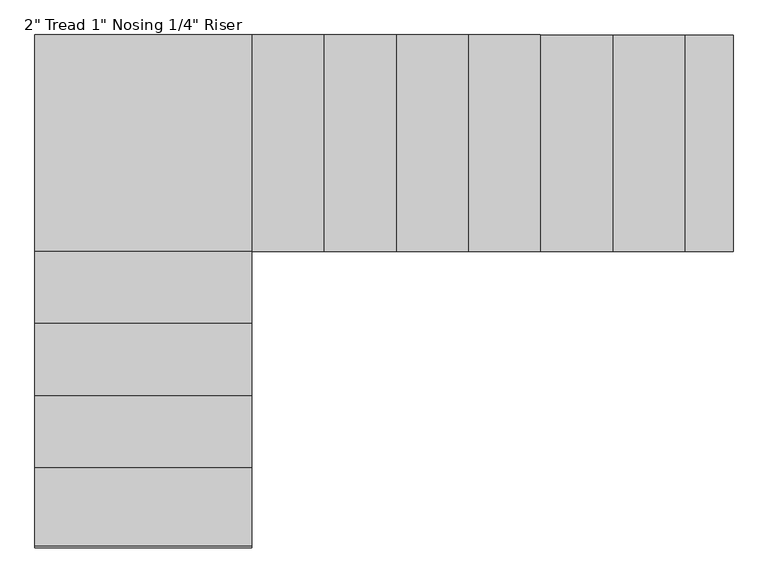
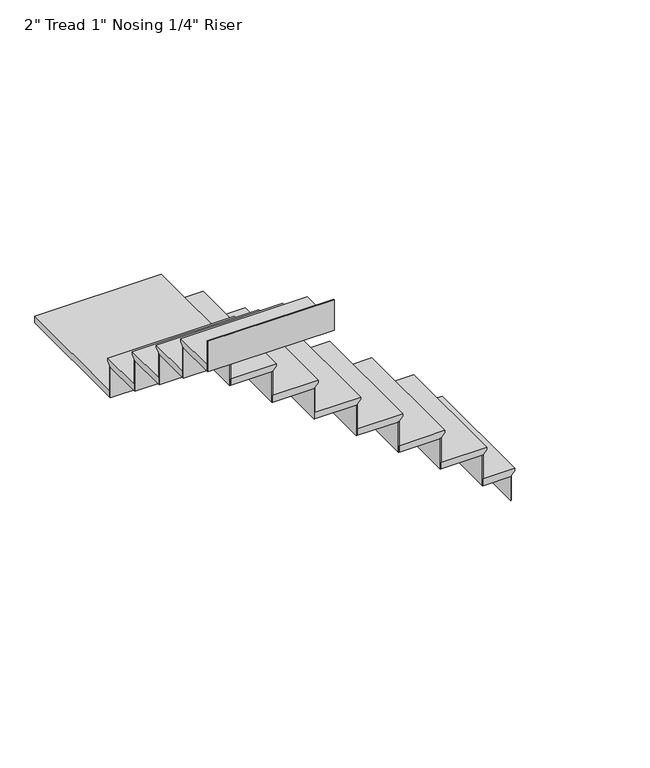
"""IFC4 building model written with IfcOpenShell, lengths in millimetres: stair flight geometry."""

from ifc_helpers import new_model, si_unit, origin, place, context, project, spatial, faceted_brep, source, transform, mapped, element, save


def stair_flight_e32d701a(model_context):
    return source(origin(), model_context, "Body", "Brep", [
        faceted_brep([(-442.4415084, 5282.3381995, 215.4115385), (-442.4415084, 5282.3381995, 234.4615385), (-442.4415084, 4368.3146777, 234.4615385), (-442.4415084, 4368.3146777, 215.4115385), (-467.8415084, 5282.3381995, 190.0115385), (-467.8415084, 4368.3146777, 190.0115385), (-671.0415084, 5282.3381995, 234.4615385), (-671.0415084, 4368.3146777, 234.4615385), (-467.8415084, 4368.3146777, 183.6615385), (-671.0415084, 4368.3146777, 183.6615385), (-671.0415084, 5282.3381995, 183.6615385), (-467.8415084, 5282.3381995, 183.6615385)], [[[0, 1, 2, 3]], [[4, 0, 3, 5]], [[2, 1, 6, 7]], [[8, 9, 10, 11]], [[2, 7, 9, 8, 5, 3]], [[8, 11, 4, 5]], [[6, 1, 0, 4, 11, 10]], [[7, 6, 10, 9]]]),
        faceted_brep([(-467.8415084, 5282.3381995, 183.6615385), (-467.8415084, 5282.3381995, 0.0), (-474.1915084, 5282.3381995, 0.0), (-474.1915084, 5282.3381995, 183.6615385), (-467.8415084, 4368.3146777, 183.6615385), (-474.1915084, 4368.3146777, 183.6615385), (-474.1915084, 4368.3146777, 0.0), (-467.8415084, 4368.3146777, 0.0)], [[[0, 1, 2, 3]], [[4, 5, 6, 7]], [[1, 0, 4, 7]], [[2, 1, 7, 6]], [[3, 2, 6, 5]], [[0, 3, 5, 4]]]),
        faceted_brep([(-671.0415084, 5282.3381995, 418.1230769), (-671.0415084, 5282.3381995, 183.6615385), (-677.3915084, 5282.3381995, 183.6615385), (-677.3915084, 5282.3381995, 418.1230769), (-671.0415084, 4368.3146777, 418.1230769), (-677.3915084, 4368.3146777, 418.1230769), (-677.3915084, 4368.3146777, 183.6615385), (-671.0415084, 4368.3146777, 183.6615385)], [[[0, 1, 2, 3]], [[4, 5, 6, 7]], [[1, 0, 4, 7]], [[2, 1, 7, 6]], [[3, 2, 6, 5]], [[0, 3, 5, 4]]]),
        faceted_brep([(-645.6415084, 4368.3146777, 468.9230769), (-645.6415084, 5282.3381995, 468.9230769), (-975.8415084, 5282.3381995, 468.9230769), (-975.8415084, 4368.3146777, 468.9230769), (-671.0415084, 4368.3146777, 418.1230769), (-975.8415084, 4368.3146777, 418.1230769), (-975.8415084, 5282.3381995, 418.1230769), (-671.0415084, 5282.3381995, 418.1230769), (-671.0415084, 4368.3146777, 424.4730769), (-645.6415084, 4368.3146777, 449.8730769), (-671.0415084, 5282.3381995, 424.4730769), (-645.6415084, 5282.3381995, 449.8730769)], [[[0, 1, 2, 3]], [[4, 5, 6, 7]], [[0, 3, 5, 4, 8, 9]], [[4, 7, 10, 8]], [[2, 1, 11, 10, 7, 6]], [[3, 2, 6, 5]], [[11, 1, 0, 9]], [[10, 11, 9, 8]]]),
        faceted_brep([(-975.8415084, 5282.3381995, 652.5846154), (-975.8415084, 5282.3381995, 418.1230769), (-982.1915084, 5282.3381995, 418.1230769), (-982.1915084, 5282.3381995, 652.5846154), (-975.8415084, 4368.3146777, 652.5846154), (-982.1915084, 4368.3146777, 652.5846154), (-982.1915084, 4368.3146777, 418.1230769), (-975.8415084, 4368.3146777, 418.1230769)], [[[0, 1, 2, 3]], [[4, 5, 6, 7]], [[1, 0, 4, 7]], [[2, 1, 7, 6]], [[3, 2, 6, 5]], [[0, 3, 5, 4]]]),
        faceted_brep([(-950.4415084, 4368.3146777, 703.3846154), (-950.4415084, 5282.3381995, 703.3846154), (-1280.6415084, 5282.3381995, 703.3846154), (-1280.6415084, 4368.3146777, 703.3846154), (-975.8415084, 4368.3146777, 652.5846154), (-1280.6415084, 4368.3146777, 652.5846154), (-1280.6415084, 5282.3381995, 652.5846154), (-975.8415084, 5282.3381995, 652.5846154), (-975.8415084, 4368.3146777, 658.9346154), (-950.4415084, 4368.3146777, 684.3346154), (-975.8415084, 5282.3381995, 658.9346154), (-950.4415084, 5282.3381995, 684.3346154)], [[[0, 1, 2, 3]], [[4, 5, 6, 7]], [[0, 3, 5, 4, 8, 9]], [[4, 7, 10, 8]], [[2, 1, 11, 10, 7, 6]], [[3, 2, 6, 5]], [[11, 1, 0, 9]], [[10, 11, 9, 8]]]),
        faceted_brep([(-1280.6415084, 5282.3381995, 887.0461538), (-1280.6415084, 5282.3381995, 652.5846154), (-1286.9915084, 5282.3381995, 652.5846154), (-1286.9915084, 5282.3381995, 887.0461538), (-1280.6415084, 4368.3146777, 887.0461538), (-1286.9915084, 4368.3146777, 887.0461538), (-1286.9915084, 4368.3146777, 652.5846154), (-1280.6415084, 4368.3146777, 652.5846154)], [[[0, 1, 2, 3]], [[4, 5, 6, 7]], [[1, 0, 4, 7]], [[2, 1, 7, 6]], [[3, 2, 6, 5]], [[0, 3, 5, 4]]]),
        faceted_brep([(-1255.2415084, 4368.3146777, 937.8461538), (-1255.2415084, 5282.3381995, 937.8461538), (-1585.4415084, 5282.3381995, 937.8461538), (-1585.4415084, 4368.3146777, 937.8461538), (-1280.6415084, 4368.3146777, 887.0461538), (-1585.4415084, 4368.3146777, 887.0461538), (-1585.4415084, 5282.3381995, 887.0461538), (-1280.6415084, 5282.3381995, 887.0461538), (-1280.6415084, 4368.3146777, 893.3961538), (-1255.2415084, 4368.3146777, 918.7961538), (-1280.6415084, 5282.3381995, 893.3961538), (-1255.2415084, 5282.3381995, 918.7961538)], [[[0, 1, 2, 3]], [[4, 5, 6, 7]], [[0, 3, 5, 4, 8, 9]], [[4, 7, 10, 8]], [[2, 1, 11, 10, 7, 6]], [[3, 2, 6, 5]], [[11, 1, 0, 9]], [[10, 11, 9, 8]]]),
        faceted_brep([(-1585.4415084, 5282.3381995, 1121.5076923), (-1585.4415084, 5282.3381995, 887.0461538), (-1591.7915084, 5282.3381995, 887.0461538), (-1591.7915084, 5282.3381995, 1121.5076923), (-1585.4415084, 4368.3146777, 1121.5076923), (-1591.7915084, 4368.3146777, 1121.5076923), (-1591.7915084, 4368.3146777, 887.0461538), (-1585.4415084, 4368.3146777, 887.0461538)], [[[0, 1, 2, 3]], [[4, 5, 6, 7]], [[1, 0, 4, 7]], [[2, 1, 7, 6]], [[3, 2, 6, 5]], [[0, 3, 5, 4]]]),
        faceted_brep([(-1560.0415084, 4368.3146777, 1172.3076923), (-1560.0415084, 5282.3381995, 1172.3076923), (-1890.2415084, 5282.3381995, 1172.3076923), (-1890.2415084, 4368.3146777, 1172.3076923), (-1585.4415084, 4368.3146777, 1121.5076923), (-1890.2415084, 4368.3146777, 1121.5076923), (-1890.2415084, 5282.3381995, 1121.5076923), (-1585.4415084, 5282.3381995, 1121.5076923), (-1585.4415084, 4368.3146777, 1127.8576923), (-1560.0415084, 4368.3146777, 1153.2576923), (-1585.4415084, 5282.3381995, 1127.8576923), (-1560.0415084, 5282.3381995, 1153.2576923)], [[[0, 1, 2, 3]], [[4, 5, 6, 7]], [[0, 3, 5, 4, 8, 9]], [[4, 7, 10, 8]], [[2, 1, 11, 10, 7, 6]], [[3, 2, 6, 5]], [[11, 1, 0, 9]], [[10, 11, 9, 8]]]),
        faceted_brep([(-1890.2415084, 5282.3381995, 1355.9692308), (-1890.2415084, 5282.3381995, 1121.5076923), (-1896.5915084, 5282.3381995, 1121.5076923), (-1896.5915084, 5282.3381995, 1355.9692308), (-1890.2415084, 4368.3146777, 1355.9692308), (-1896.5915084, 4368.3146777, 1355.9692308), (-1896.5915084, 4368.3146777, 1121.5076923), (-1890.2415084, 4368.3146777, 1121.5076923)], [[[0, 1, 2, 3]], [[4, 5, 6, 7]], [[1, 0, 4, 7]], [[2, 1, 7, 6]], [[3, 2, 6, 5]], [[0, 3, 5, 4]]]),
        faceted_brep([(-1864.8415084, 4368.3146777, 1406.7692308), (-1864.8415084, 5282.3381995, 1406.7692308), (-2195.0415084, 5282.3381995, 1406.7692308), (-2195.0415084, 4368.3146777, 1406.7692308), (-1890.2415084, 4368.3146777, 1355.9692308), (-2195.0415084, 4368.3146777, 1355.9692308), (-2195.0415084, 5282.3381995, 1355.9692308), (-1890.2415084, 5282.3381995, 1355.9692308), (-1890.2415084, 4368.3146777, 1362.3192308), (-1864.8415084, 4368.3146777, 1387.7192308), (-1890.2415084, 5282.3381995, 1362.3192308), (-1864.8415084, 5282.3381995, 1387.7192308)], [[[0, 1, 2, 3]], [[4, 5, 6, 7]], [[0, 3, 5, 4, 8, 9]], [[4, 7, 10, 8]], [[2, 1, 11, 10, 7, 6]], [[3, 2, 6, 5]], [[11, 1, 0, 9]], [[10, 11, 9, 8]]]),
        faceted_brep([(-2195.0415084, 5282.3381995, 1590.4307692), (-2195.0415084, 5282.3381995, 1355.9692308), (-2201.3915084, 5282.3381995, 1355.9692308), (-2201.3915084, 5282.3381995, 1590.4307692), (-2195.0415084, 4368.3146777, 1590.4307692), (-2201.3915084, 4368.3146777, 1590.4307692), (-2201.3915084, 4368.3146777, 1355.9692308), (-2195.0415084, 4368.3146777, 1355.9692308)], [[[0, 1, 2, 3]], [[4, 5, 6, 7]], [[1, 0, 4, 7]], [[2, 1, 7, 6]], [[3, 2, 6, 5]], [[0, 3, 5, 4]]]),
        faceted_brep([(-2169.6415084, 4368.3146777, 1641.2307692), (-2169.6415084, 5282.3381995, 1641.2307692), (-2499.8415084, 5282.3381995, 1641.2307692), (-2499.8415084, 4368.3146777, 1641.2307692), (-2195.0415084, 4368.3146777, 1590.4307692), (-2499.8415084, 4368.3146777, 1590.4307692), (-2499.8415084, 5282.3381995, 1590.4307692), (-2195.0415084, 5282.3381995, 1590.4307692), (-2195.0415084, 4368.3146777, 1596.7807692), (-2169.6415084, 4368.3146777, 1622.1807692), (-2195.0415084, 5282.3381995, 1596.7807692), (-2169.6415084, 5282.3381995, 1622.1807692)], [[[0, 1, 2, 3]], [[4, 5, 6, 7]], [[0, 3, 5, 4, 8, 9]], [[4, 7, 10, 8]], [[2, 1, 11, 10, 7, 6]], [[3, 2, 6, 5]], [[11, 1, 0, 9]], [[10, 11, 9, 8]]]),
        faceted_brep([(-2499.8415084, 5282.3381995, 1824.8923077), (-2499.8415084, 5282.3381995, 1590.4307692), (-2506.1915084, 5282.3381995, 1590.4307692), (-2506.1915084, 5282.3381995, 1824.8923077), (-2499.8415084, 4368.3146777, 1824.8923077), (-2506.1915084, 4368.3146777, 1824.8923077), (-2506.1915084, 4368.3146777, 1590.4307692), (-2499.8415084, 4368.3146777, 1590.4307692)], [[[0, 1, 2, 3]], [[4, 5, 6, 7]], [[1, 0, 4, 7]], [[2, 1, 7, 6]], [[3, 2, 6, 5]], [[0, 3, 5, 4]]]),
        faceted_brep([(-3388.8415084, 5282.3381995, 1875.6923077), (-3388.8415084, 4342.9146777, 1875.6923077), (-2474.4415084, 4342.9146777, 1875.6923077), (-2474.4415084, 5282.3381995, 1875.6923077), (-2474.4415084, 4368.3146777, 1824.8923077), (-2474.4415084, 4342.9146777, 1824.8923077), (-3388.8415084, 4342.9146777, 1824.8923077), (-3388.8415084, 5282.3381995, 1824.8923077), (-2499.8415084, 5282.3381995, 1824.8923077), (-2499.8415084, 4368.3146777, 1824.8923077), (-2474.4415084, 4368.3146777, 1856.6423077), (-2474.4415084, 5282.3381995, 1856.6423077), (-2499.8415084, 4368.3146777, 1831.2423077), (-2499.8415084, 5282.3381995, 1831.2423077)], [[[0, 1, 2, 3]], [[4, 5, 6, 7, 8, 9]], [[3, 2, 5, 4, 10, 11]], [[4, 9, 12, 10]], [[9, 8, 13, 12]], [[0, 3, 11, 13, 8, 7]], [[1, 0, 7, 6]], [[2, 1, 6, 5]], [[13, 11, 10, 12]]]),
        faceted_brep([(-3388.8415084, 4342.9146777, 2059.3538462), (-3388.8415084, 4342.9146777, 1824.8923077), (-3388.8415084, 4336.5646777, 1824.8923077), (-3388.8415084, 4336.5646777, 2059.3538462), (-2474.4415084, 4342.9146777, 2059.3538462), (-2474.4415084, 4336.5646777, 2059.3538462), (-2474.4415084, 4336.5646777, 1824.8923077), (-2474.4415084, 4342.9146777, 1824.8923077)], [[[0, 1, 2, 3]], [[4, 5, 6, 7]], [[1, 0, 4, 7]], [[2, 1, 7, 6]], [[3, 2, 6, 5]], [[0, 3, 5, 4]]]),
        faceted_brep([(-2474.4415084, 4368.3146777, 2110.1538462), (-3388.8415084, 4368.3146777, 2110.1538462), (-3388.8415084, 4037.7382512, 2110.1538462), (-2474.4415084, 4037.7382512, 2110.1538462), (-2474.4415084, 4342.9146777, 2059.3538462), (-2474.4415084, 4037.7382512, 2059.3538462), (-3388.8415084, 4037.7382512, 2059.3538462), (-3388.8415084, 4342.9146777, 2059.3538462), (-2474.4415084, 4342.9146777, 2065.7038462), (-2474.4415084, 4368.3146777, 2091.1038462), (-3388.8415084, 4342.9146777, 2065.7038462), (-3388.8415084, 4368.3146777, 2091.1038462)], [[[0, 1, 2, 3]], [[4, 5, 6, 7]], [[0, 3, 5, 4, 8, 9]], [[4, 7, 10, 8]], [[2, 1, 11, 10, 7, 6]], [[3, 2, 6, 5]], [[11, 1, 0, 9]], [[10, 11, 9, 8]]]),
        faceted_brep([(-3388.8415084, 4037.7382512, 2293.8153846), (-3388.8415084, 4037.7382512, 2059.3538462), (-3388.8415084, 4031.3882512, 2059.3538462), (-3388.8415084, 4031.3882512, 2293.8153846), (-2474.4415084, 4037.7382512, 2293.8153846), (-2474.4415084, 4031.3882512, 2293.8153846), (-2474.4415084, 4031.3882512, 2059.3538462), (-2474.4415084, 4037.7382512, 2059.3538462)], [[[0, 1, 2, 3]], [[4, 5, 6, 7]], [[1, 0, 4, 7]], [[2, 1, 7, 6]], [[3, 2, 6, 5]], [[0, 3, 5, 4]]]),
        faceted_brep([(-2474.4415084, 4063.1382512, 2344.6153846), (-3388.8415084, 4063.1382512, 2344.6153846), (-3388.8415084, 3732.938277, 2344.6153846), (-2474.4415084, 3732.938277, 2344.6153846), (-2474.4415084, 4037.7382512, 2293.8153846), (-2474.4415084, 3732.938277, 2293.8153846), (-3388.8415084, 3732.938277, 2293.8153846), (-3388.8415084, 4037.7382512, 2293.8153846), (-2474.4415084, 4037.7382512, 2300.1653846), (-2474.4415084, 4063.1382512, 2325.5653846), (-3388.8415084, 4037.7382512, 2300.1653846), (-3388.8415084, 4063.1382512, 2325.5653846)], [[[0, 1, 2, 3]], [[4, 5, 6, 7]], [[0, 3, 5, 4, 8, 9]], [[4, 7, 10, 8]], [[2, 1, 11, 10, 7, 6]], [[3, 2, 6, 5]], [[11, 1, 0, 9]], [[10, 11, 9, 8]]]),
        faceted_brep([(-3388.8415084, 3732.938277, 2528.2769231), (-3388.8415084, 3732.938277, 2293.8153846), (-3388.8415084, 3726.588277, 2293.8153846), (-3388.8415084, 3726.588277, 2528.2769231), (-2474.4415084, 3732.938277, 2528.2769231), (-2474.4415084, 3726.588277, 2528.2769231), (-2474.4415084, 3726.588277, 2293.8153846), (-2474.4415084, 3732.938277, 2293.8153846)], [[[0, 1, 2, 3]], [[4, 5, 6, 7]], [[1, 0, 4, 7]], [[2, 1, 7, 6]], [[3, 2, 6, 5]], [[0, 3, 5, 4]]]),
        faceted_brep([(-2474.4415084, 3758.338277, 2579.0769231), (-3388.8415084, 3758.338277, 2579.0769231), (-3388.8415084, 3428.1383028, 2579.0769231), (-2474.4415084, 3428.1383028, 2579.0769231), (-2474.4415084, 3732.938277, 2528.2769231), (-2474.4415084, 3428.1383028, 2528.2769231), (-3388.8415084, 3428.1383028, 2528.2769231), (-3388.8415084, 3732.938277, 2528.2769231), (-2474.4415084, 3732.938277, 2534.6269231), (-2474.4415084, 3758.338277, 2560.0269231), (-3388.8415084, 3732.938277, 2534.6269231), (-3388.8415084, 3758.338277, 2560.0269231)], [[[0, 1, 2, 3]], [[4, 5, 6, 7]], [[0, 3, 5, 4, 8, 9]], [[4, 7, 10, 8]], [[2, 1, 11, 10, 7, 6]], [[3, 2, 6, 5]], [[11, 1, 0, 9]], [[10, 11, 9, 8]]]),
        faceted_brep([(-3388.8415084, 3428.1383028, 2762.7384615), (-3388.8415084, 3428.1383028, 2528.2769231), (-3388.8415084, 3421.7883028, 2528.2769231), (-3388.8415084, 3421.7883028, 2762.7384615), (-2474.4415084, 3428.1383028, 2762.7384615), (-2474.4415084, 3421.7883028, 2762.7384615), (-2474.4415084, 3421.7883028, 2528.2769231), (-2474.4415084, 3428.1383028, 2528.2769231)], [[[0, 1, 2, 3]], [[4, 5, 6, 7]], [[1, 0, 4, 7]], [[2, 1, 7, 6]], [[3, 2, 6, 5]], [[0, 3, 5, 4]]]),
        faceted_brep([(-3388.8415084, 3123.3383287, 2997.2), (-3388.8415084, 3123.3383287, 2762.7384615), (-3388.8415084, 3116.9883287, 2762.7384615), (-3388.8415084, 3116.9883287, 2997.2), (-2474.4415084, 3123.3383287, 2997.2), (-2474.4415084, 3116.9883287, 2997.2), (-2474.4415084, 3116.9883287, 2762.7384615), (-2474.4415084, 3123.3383287, 2762.7384615)], [[[0, 1, 2, 3]], [[4, 5, 6, 7]], [[1, 0, 4, 7]], [[2, 1, 7, 6]], [[3, 2, 6, 5]], [[0, 3, 5, 4]]]),
        faceted_brep([(-2474.4415084, 3453.5383028, 2813.5384615), (-3388.8415084, 3453.5383028, 2813.5384615), (-3388.8415084, 3123.3383287, 2813.5384615), (-2474.4415084, 3123.3383287, 2813.5384615), (-2474.4415084, 3428.1383028, 2762.7384615), (-2474.4415084, 3123.3383287, 2762.7384615), (-3388.8415084, 3123.3383287, 2762.7384615), (-3388.8415084, 3428.1383028, 2762.7384615), (-2474.4415084, 3428.1383028, 2769.0884615), (-2474.4415084, 3453.5383028, 2794.4884615), (-3388.8415084, 3428.1383028, 2769.0884615), (-3388.8415084, 3453.5383028, 2794.4884615)], [[[0, 1, 2, 3]], [[4, 5, 6, 7]], [[0, 3, 5, 4, 8, 9]], [[4, 7, 10, 8]], [[2, 1, 11, 10, 7, 6]], [[3, 2, 6, 5]], [[11, 1, 0, 9]], [[10, 11, 9, 8]]]),
    ])


if __name__ == "__main__":
    model = new_model("IFC4")
    model_context = context("Model", 3, world=origin())
    ifc_project = project(units=[si_unit("LENGTHUNIT", "METRE", prefix="MILLI")], contexts=[model_context])
    site = spatial("IfcSite", under=ifc_project)
    building = spatial("IfcBuilding", under=site)
    placement = place(None, origin())
    stair_flight_shape = stair_flight_e32d701a(model_context)
    element("IfcStairFlight", 1, ObjectType="2\" Tread 1\" Nosing 1/4\" Riser", at=placement, inside=building, context=model_context, shape_type="MappedRepresentation", body=[
        mapped(stair_flight_shape, transform((0.0, 0.0, 0.0), x_axis=(1.0, 0.0, 0.0), y_axis=(0.0, 1.0, 0.0), z_axis=(0.0, 0.0, 1.0))),
    ])
    save(model, "model.ifc")
